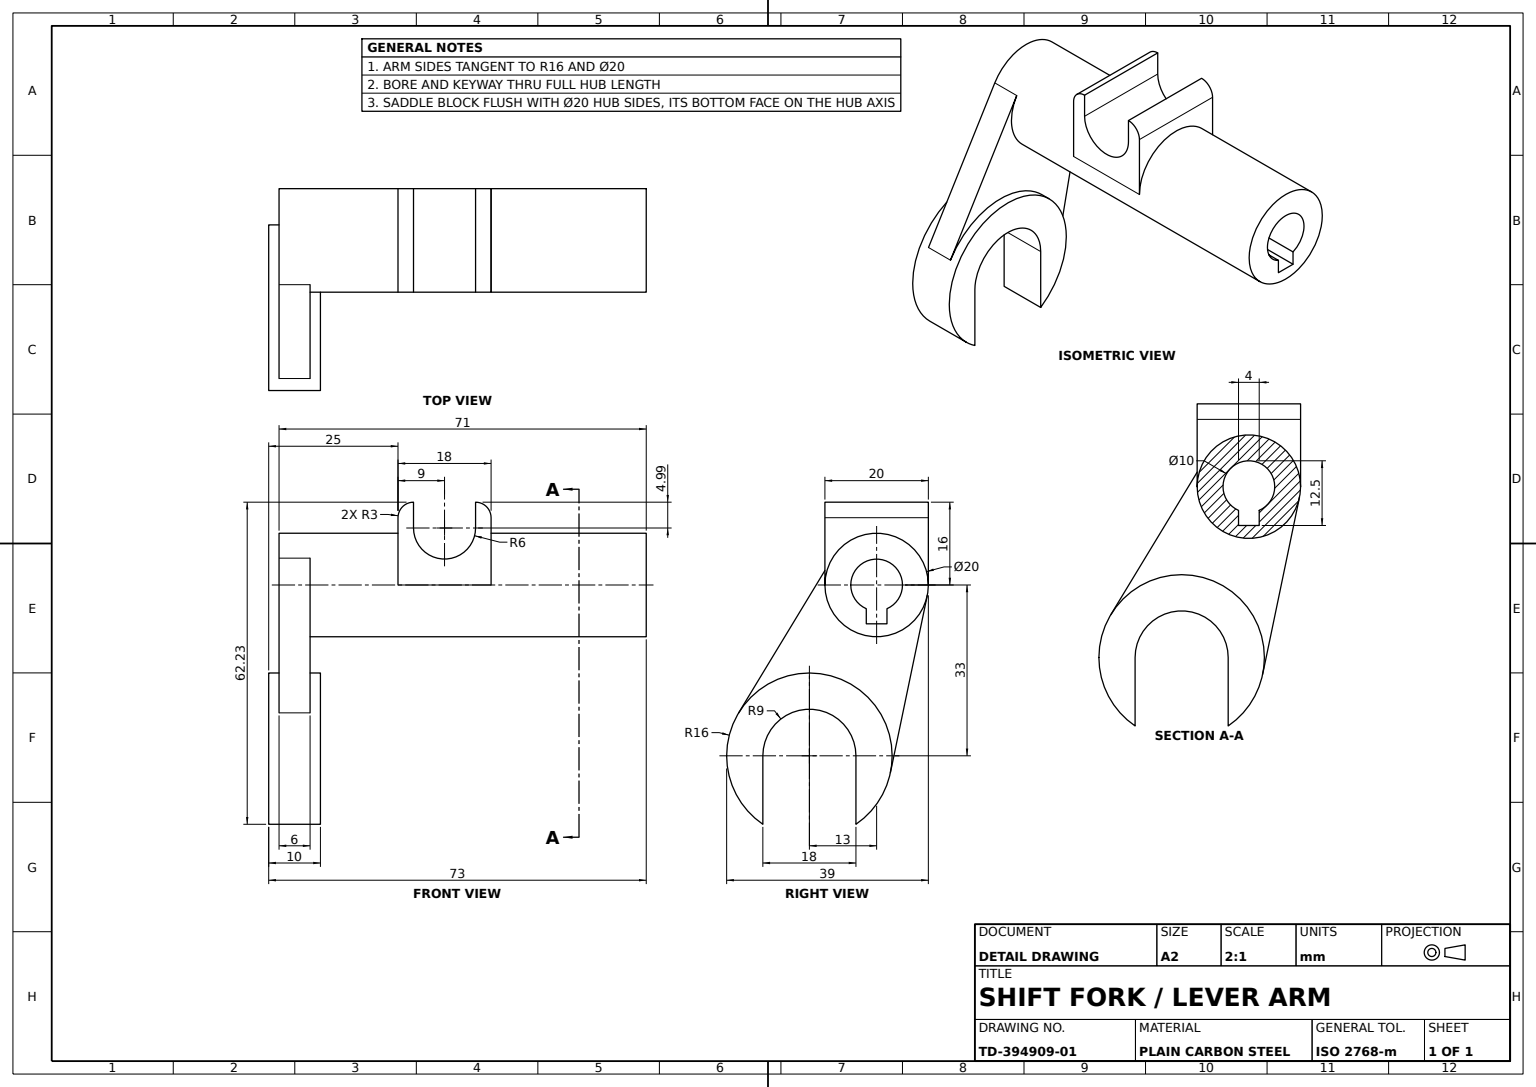
SolidWorks part; units mm, degrees
material "Plain Carbon Steel"
ref_plane "Front Plane" through (0, 0, 0) normal (0, 0, 1) x (1, 0, 0)
ref_plane "Top Plane" through (0, 0, 0) normal (0, 1, 0) x (1, 0, 0)
ref_plane "Right Plane" through (0, 0, 0) normal (1, 0, 0) x (0, 0, -1)
sketch "Hub Profile Ø20" plane through (0, 0, 0) normal (1, 0, 0) x (0, 0, -1)
  circle A0 centre (0, 0) radius 10
  dimension "D1" = 20
extrude "Shaft Hub Ø20x71" add sketch "Hub Profile Ø20" along normal blind 71
sketch "Keyed Bore Profile" plane through (71, 0, 0) normal (1, 0, 0) x (0, 0, -1)
  line L0 (-2, -4.5826) -> (-2, -7.5)
  line L1 (-2, -7.5) -> (2, -7.5)
  line L2 (2, -7.5) -> (2, -4.5826)
  arc A0 (2, -4.5826) -> (-2, -4.5826) centre (0, 0) ccw
  point P1 (0, -7.5)
  point P5 (0, 5)
  dimension "D1" = 10
  dimension "D2" = 12.5
  dimension "D3" = 4
extrude "Keyed Bore Ø10" cut sketch "Keyed Bore Profile" against normal up to next
sketch "Rocker Arm Profile" plane through (71, 0, 0) normal (1, 0, 0) x (0, 0, -1)
  line L0 (-10, 0) -> (-10, 16)
  line L1 (-10, 16) -> (10, 16)
  line L2 (10, 16) -> (10, 0)
  line L3 (-10, 0) -> (10, 0) construction
  circle A0 centre (0, 0) radius 10 construction
  arc A1 (10, 0) -> (-10, 0) centre (0, 0) ccw
  dimension "D1" = 16
extrude "Rocker Arm" add sketch "Rocker Arm Profile" against normal blind 18 from offset 30 offset against normal yes
fillet "Arm Fillet R3" radius 3 2 edges at (23, 16, 0) (41, 16, 0)
sketch "Fork Slot Profile" plane through (0, 0, 0) normal (0, 0, 1) x (1, 0, 0)
  line L5 (26, 16) -> (26, 11.01)
  line L6 (38, 11.01) -> (38, 16)
  line L8 (26, 16) -> (38, 16)
  line L9 (26, 16) -> (38, 16) construction
  line L10 (23, 0) -> (41, 0) construction
  arc A1 (26, 11.01) -> (38, 11.01) centre (32, 11.01) ccw
  point P5 (32, 0)
  dimension "D1" = 4.99
  dimension "D2" = 6
sketch "Saddle Block Profile" plane through (0, 0, 0) normal (-1, 0, 0) x (0, 0, 1)
  line L0 (22, -33) -> (22, -46.2288)
  line L1 (4, -33) -> (4, -46.2288)
  line L2 (0, 0) -> (13, 0) construction
  line L3 (13, 0) -> (13, -33) construction
  arc A0 (22, -46.2288) -> (4, -46.2288) centre (13, -33) ccw
  arc A1 (22, -33) -> (4, -33) centre (13, -33) ccw
  dimension "D1" = 16
  dimension "D2" = 9
  dimension "D3" = 13
  dimension "D4" = 33
extrude "Saddle Block" add sketch "Saddle Block Profile" against normal blind 8 and the other way blind 2 separate body
sketch "Connecting Web Profile" plane through (0, 0, 0) normal (-1, 0, 0) x (0, 0, 1)
  line L0 (26.6799, -24.7018) -> (8.55, 5.1863)
  line L1 (-2.664, -36.2616) -> (-9.79, -2.0385)
  arc A0 (22, -46.2288) -> (4, -46.2288) centre (13, -33) ccw construction
  arc A1 (10, 0) -> (-10, 0) centre (0, 0) ccw construction
  circle A2 centre (0, 0) radius 10 construction
  arc A3 (26.6799, -24.7018) -> (-2.664, -36.2616) centre (13, -33) ccw
  arc A4 (-9.79, -2.0385) -> (8.55, 5.1863) centre (0, 0) ccw
  arc A5 (-9.79, -2.0385) -> (8.55, 5.1863) centre (0, 0) ccw
  circle M7 centre (0, 0) radius 10
extrude "Connecting Web" add sketch "Connecting Web Profile" against normal blind 6 contours A3 L0 L1 M7
extrude "Fork Slot" cut sketch "Fork Slot Profile" against normal through all both and the other way through all
